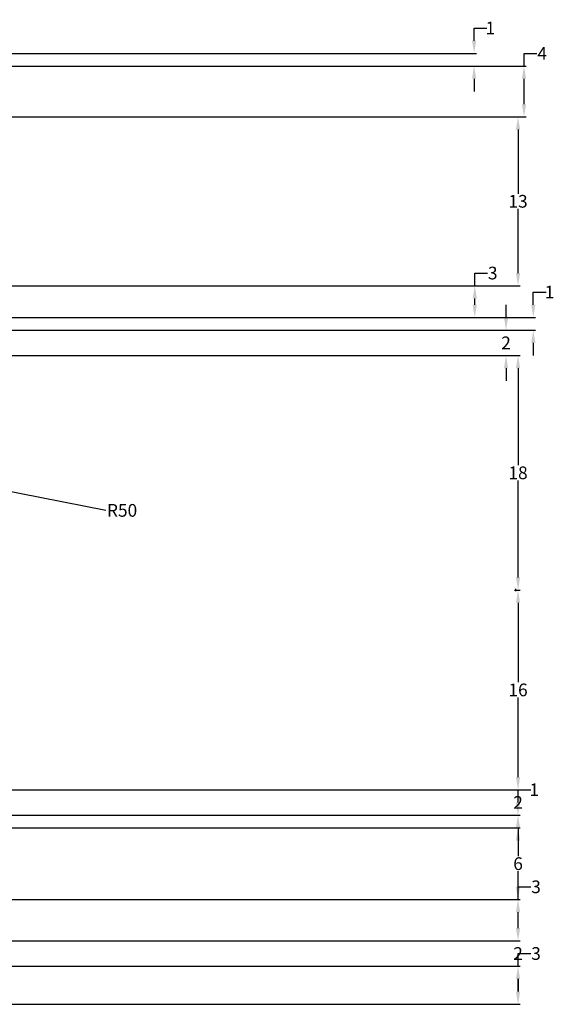
# Model space of a CAD drawing. Units: millimetres. Extents: x 31 to 232, y 35 to 192.
# Tile 3 of 5: x 80 to 122, y 43 to 121. Entities that reach past the tile are written whole.
import ezdxf

# ---------------------------------------------------------------- set-up
doc = ezdxf.new("R2010")
doc.units = ezdxf.units.MM
doc.header["$MEASUREMENT"] = 0
doc.layers.add('M-DIMS', color=2, linetype='Continuous', lineweight=25)
doc.styles.get("Standard").update_dxf_attribs({"font": 'arial.ttf'})
doc.dimstyles.get("Standard").update_dxf_attribs({"dimtxt": 1, "dimasz": 1, "dimexe": 0.18, "dimexo": 0.0625, "dimgap": 0.09, "dimtad": 0, "dimtih": 1, "dimtoh": 1, "dimdec": 0, "dimzin": 0, "dimdsep": 46, "dimtxsty": 'Standard', "dimcen": 0.09, "dimadec": 0, "dimazin": 0, "dimtfac": 1, "dimtdec": 0, "dimtofl": 0, "dimtmove": 0, "dimatfit": 3, "dimfxl": 1, "dimtolj": 1, "dimtzin": 0, "dimarcsym": 0})

# ---------------------------------------------------------------- blocks, each defined once
blk = doc.blocks.new('*D4')
at = {"layer": 'Defpoints', "color": 0, "transparency": 16777216}
for p in [(78.774, 46.183), (119.423, 46.183), (78.774, 43.183)]:
    blk.add_point(p, dxfattribs=at)
at = {"layer": 'M-DIMS', "color": 0, "lineweight": -2, "transparency": 16777216}
for p, q in [((119.423, 46.183), (119.423, 47.183)), ((119.423, 47.183), (120.423, 47.183)), ((78.836, 46.183), (119.603, 46.183)), ((119.423, 44.183), (119.423, 45.183)), ((78.836, 43.183), (119.603, 43.183))]:
    blk.add_line(p, q, dxfattribs=at)
at = {"layer": 'M-DIMS', "color": 0, "transparency": 16777216}
for points in [[(119.256, 45.183), (119.589, 45.183), (119.423, 46.183)], [(119.256, 44.183), (119.589, 44.183), (119.423, 43.183)]]:
    blk.add_solid(points, dxfattribs=at)
at = {"layer": 'M-DIMS', "color": 0, "transparency": 16777216, "insert": (120.84, 47.183), "char_height": 1, "attachment_point": 5}
blk.add_mtext('\\A1;3', dxfattribs=at)
blk = doc.blocks.new('*D5')
at = {"layer": 'Defpoints', "color": 0, "transparency": 16777216}
for p in [(76.774, 48.183), (119.423, 48.183), (78.774, 46.183)]:
    blk.add_point(p, dxfattribs=at)
at = {"layer": 'M-DIMS', "color": 0, "lineweight": -2, "transparency": 16777216}
for p, q in [((119.423, 49.183), (119.423, 50.183)), ((76.836, 48.183), (119.603, 48.183)), ((78.836, 46.183), (119.603, 46.183)), ((119.423, 45.183), (119.423, 44.183))]:
    blk.add_line(p, q, dxfattribs=at)
at = {"layer": 'M-DIMS', "color": 0, "transparency": 16777216}
for points in [[(119.256, 49.183), (119.589, 49.183), (119.423, 48.183)], [(119.256, 45.183), (119.589, 45.183), (119.423, 46.183)]]:
    blk.add_solid(points, dxfattribs=at)
at = {"layer": 'M-DIMS', "color": 0, "transparency": 16777216, "insert": (119.423, 47.183), "char_height": 1, "attachment_point": 5}
blk.add_mtext('\\A1;2', dxfattribs=at)
blk = doc.blocks.new('*D6')
at = {"layer": 'Defpoints', "color": 0, "transparency": 16777216}
for p in [(77.735, 51.44), (119.423, 51.44), (76.774, 48.183)]:
    blk.add_point(p, dxfattribs=at)
at = {"layer": 'M-DIMS', "color": 0, "lineweight": -2, "transparency": 16777216}
for p, q in [((119.423, 51.44), (119.423, 52.44)), ((119.423, 52.44), (120.423, 52.44)), ((77.797, 51.44), (119.603, 51.44)), ((119.423, 49.183), (119.423, 50.44)), ((76.836, 48.183), (119.603, 48.183))]:
    blk.add_line(p, q, dxfattribs=at)
at = {"layer": 'M-DIMS', "color": 0, "transparency": 16777216}
for points in [[(119.256, 50.44), (119.589, 50.44), (119.423, 51.44)], [(119.256, 49.183), (119.589, 49.183), (119.423, 48.183)]]:
    blk.add_solid(points, dxfattribs=at)
at = {"layer": 'M-DIMS', "color": 0, "transparency": 16777216, "insert": (120.84, 52.44), "char_height": 1, "attachment_point": 5}
blk.add_mtext('\\A1;3', dxfattribs=at)
blk = doc.blocks.new('*D7')
at = {"layer": 'Defpoints', "color": 0, "transparency": 16777216}
for p in [(73.774, 57.083), (119.423, 57.083), (77.735, 51.44)]:
    blk.add_point(p, dxfattribs=at)
at = {"layer": 'M-DIMS', "color": 0, "lineweight": -2, "transparency": 16777216}
for p, q in [((73.836, 57.083), (119.603, 57.083)), ((119.423, 56.083), (119.423, 54.862)), ((119.423, 52.44), (119.423, 53.661)), ((77.797, 51.44), (119.603, 51.44))]:
    blk.add_line(p, q, dxfattribs=at)
at = {"layer": 'M-DIMS', "color": 0, "transparency": 16777216}
for points in [[(119.256, 56.083), (119.589, 56.083), (119.423, 57.083)], [(119.256, 52.44), (119.589, 52.44), (119.423, 51.44)]]:
    blk.add_solid(points, dxfattribs=at)
at = {"layer": 'M-DIMS', "color": 0, "transparency": 16777216, "insert": (119.423, 54.261), "char_height": 1, "attachment_point": 5}
blk.add_mtext('\\A1;6', dxfattribs=at)
blk = doc.blocks.new('*D8')
at = {"layer": 'Defpoints', "color": 0, "transparency": 16777216}
for p in [(73.774, 58.083), (119.423, 58.083), (73.774, 57.083)]:
    blk.add_point(p, dxfattribs=at)
at = {"layer": 'M-DIMS', "color": 0, "lineweight": -2, "transparency": 16777216}
for p, q in [((119.423, 59.083), (119.423, 60.083)), ((119.423, 60.083), (120.423, 60.083)), ((73.836, 58.083), (119.603, 58.083)), ((73.836, 57.083), (119.603, 57.083)), ((119.423, 56.083), (119.423, 55.083))]:
    blk.add_line(p, q, dxfattribs=at)
at = {"layer": 'M-DIMS', "color": 0, "transparency": 16777216}
for points in [[(119.256, 59.083), (119.589, 59.083), (119.423, 58.083)], [(119.256, 56.083), (119.589, 56.083), (119.423, 57.083)]]:
    blk.add_solid(points, dxfattribs=at)
at = {"layer": 'M-DIMS', "color": 0, "transparency": 16777216, "insert": (120.697, 60.083), "char_height": 1, "attachment_point": 5}
blk.add_mtext('\\A1;1', dxfattribs=at)
blk = doc.blocks.new('*D9')
at = {"layer": 'Defpoints', "color": 0, "transparency": 16777216}
for p in [(71.774, 60.083), (119.423, 60.083), (73.774, 58.083)]:
    blk.add_point(p, dxfattribs=at)
at = {"layer": 'M-DIMS', "color": 0, "lineweight": -2, "transparency": 16777216}
for p, q in [((119.423, 61.083), (119.423, 62.083)), ((71.836, 60.083), (119.603, 60.083)), ((73.836, 58.083), (119.603, 58.083)), ((119.423, 57.083), (119.423, 56.083))]:
    blk.add_line(p, q, dxfattribs=at)
at = {"layer": 'M-DIMS', "color": 0, "transparency": 16777216}
for points in [[(119.256, 61.083), (119.589, 61.083), (119.423, 60.083)], [(119.256, 57.083), (119.589, 57.083), (119.423, 58.083)]]:
    blk.add_solid(points, dxfattribs=at)
at = {"layer": 'M-DIMS', "color": 0, "transparency": 16777216, "insert": (119.423, 59.083), "char_height": 1, "attachment_point": 5}
blk.add_mtext('\\A1;2', dxfattribs=at)
blk = doc.blocks.new('*D10')
at = {"layer": 'Defpoints', "color": 0, "transparency": 16777216}
for p in [(119.236, 75.81), (119.423, 75.81), (71.774, 60.083)]:
    blk.add_point(p, dxfattribs=at)
at = {"layer": 'M-DIMS', "color": 0, "lineweight": -2, "transparency": 16777216}
for p, q in [((119.298, 75.81), (119.603, 75.81)), ((119.423, 74.81), (119.423, 68.547)), ((119.423, 61.083), (119.423, 67.346)), ((71.836, 60.083), (119.603, 60.083))]:
    blk.add_line(p, q, dxfattribs=at)
at = {"layer": 'M-DIMS', "color": 0, "transparency": 16777216}
for points in [[(119.256, 74.81), (119.589, 74.81), (119.423, 75.81)], [(119.256, 61.083), (119.589, 61.083), (119.423, 60.083)]]:
    blk.add_solid(points, dxfattribs=at)
at = {"layer": 'M-DIMS', "color": 0, "transparency": 16777216, "insert": (119.423, 67.946), "char_height": 1, "attachment_point": 5}
blk.add_mtext('\\A1;16', dxfattribs=at)
blk = doc.blocks.new('*D11')
at = {"layer": 'Defpoints', "color": 0, "transparency": 16777216}
for p in [(72.774, 94.283), (119.423, 94.283), (119.236, 75.81)]:
    blk.add_point(p, dxfattribs=at)
at = {"layer": 'M-DIMS', "color": 0, "lineweight": -2, "transparency": 16777216}
for p, q in [((72.836, 94.283), (119.603, 94.283)), ((119.423, 93.283), (119.423, 85.647)), ((119.423, 76.81), (119.423, 84.446)), ((119.298, 75.81), (119.603, 75.81))]:
    blk.add_line(p, q, dxfattribs=at)
at = {"layer": 'M-DIMS', "color": 0, "transparency": 16777216}
for points in [[(119.256, 93.283), (119.589, 93.283), (119.423, 94.283)], [(119.256, 76.81), (119.589, 76.81), (119.423, 75.81)]]:
    blk.add_solid(points, dxfattribs=at)
at = {"layer": 'M-DIMS', "color": 0, "transparency": 16777216, "insert": (119.423, 85.046), "char_height": 1, "attachment_point": 5}
blk.add_mtext('\\A1;18', dxfattribs=at)
blk = doc.blocks.new('*D12')
at = {"layer": 'Defpoints', "color": 0, "transparency": 16777216}
for p in [(72.774, 96.283), (118.478, 96.283), (72.774, 94.283)]:
    blk.add_point(p, dxfattribs=at)
at = {"layer": 'M-DIMS', "color": 0, "lineweight": -2, "transparency": 16777216}
for p, q in [((118.478, 97.283), (118.478, 98.283)), ((72.836, 96.283), (118.658, 96.283)), ((72.836, 94.283), (118.658, 94.283)), ((118.478, 93.283), (118.478, 92.283))]:
    blk.add_line(p, q, dxfattribs=at)
at = {"layer": 'M-DIMS', "color": 0, "transparency": 16777216}
for points in [[(118.312, 97.283), (118.645, 97.283), (118.478, 96.283)], [(118.312, 93.283), (118.645, 93.283), (118.478, 94.283)]]:
    blk.add_solid(points, dxfattribs=at)
at = {"layer": 'M-DIMS', "color": 0, "transparency": 16777216, "insert": (118.478, 95.283), "char_height": 1, "attachment_point": 5}
blk.add_mtext('\\A1;2', dxfattribs=at)
blk = doc.blocks.new('*D13')
at = {"layer": 'Defpoints', "color": 0, "transparency": 16777216}
for p in [(74.506, 97.283), (120.627, 97.283), (72.774, 96.283)]:
    blk.add_point(p, dxfattribs=at)
at = {"layer": 'M-DIMS', "color": 0, "lineweight": -2, "transparency": 16777216}
for p, q in [((120.627, 98.283), (120.627, 99.283)), ((120.627, 99.283), (121.627, 99.283)), ((74.568, 97.283), (120.807, 97.283)), ((72.836, 96.283), (120.807, 96.283)), ((120.627, 95.283), (120.627, 94.283))]:
    blk.add_line(p, q, dxfattribs=at)
at = {"layer": 'M-DIMS', "color": 0, "transparency": 16777216}
for points in [[(120.46, 98.283), (120.794, 98.283), (120.627, 97.283)], [(120.46, 95.283), (120.794, 95.283), (120.627, 96.283)]]:
    blk.add_solid(points, dxfattribs=at)
at = {"layer": 'M-DIMS', "color": 0, "transparency": 16777216, "insert": (121.901, 99.283), "char_height": 1, "attachment_point": 5}
blk.add_mtext('\\A1;1', dxfattribs=at)
blk = doc.blocks.new('*D14')
at = {"layer": 'Defpoints', "color": 0, "transparency": 16777216}
for p in [(77.006, 99.783), (116.013, 99.783), (74.506, 97.283)]:
    blk.add_point(p, dxfattribs=at)
at = {"layer": 'M-DIMS', "color": 0, "lineweight": -2, "transparency": 16777216}
for p, q in [((116.013, 99.783), (116.013, 100.783)), ((116.013, 100.783), (117.013, 100.783)), ((77.068, 99.783), (116.193, 99.783)), ((116.013, 98.283), (116.013, 98.783)), ((74.568, 97.283), (116.193, 97.283))]:
    blk.add_line(p, q, dxfattribs=at)
at = {"layer": 'M-DIMS', "color": 0, "transparency": 16777216}
for points in [[(115.846, 98.783), (116.18, 98.783), (116.013, 99.783)], [(115.846, 98.283), (116.18, 98.283), (116.013, 97.283)]]:
    blk.add_solid(points, dxfattribs=at)
at = {"layer": 'M-DIMS', "color": 0, "transparency": 16777216, "insert": (117.43, 100.783), "char_height": 1, "attachment_point": 5}
blk.add_mtext('\\A1;3', dxfattribs=at)
blk = doc.blocks.new('*D15')
at = {"layer": 'Defpoints', "color": 0, "transparency": 16777216}
for p in [(77.006, 113.083), (119.423, 113.083), (77.006, 99.783)]:
    blk.add_point(p, dxfattribs=at)
at = {"layer": 'M-DIMS', "color": 0, "lineweight": -2, "transparency": 16777216}
for p, q in [((77.068, 113.083), (119.603, 113.083)), ((119.423, 112.083), (119.423, 107.034)), ((119.423, 100.783), (119.423, 105.832)), ((77.068, 99.783), (119.603, 99.783))]:
    blk.add_line(p, q, dxfattribs=at)
at = {"layer": 'M-DIMS', "color": 0, "transparency": 16777216}
for points in [[(119.256, 112.083), (119.589, 112.083), (119.423, 113.083)], [(119.256, 100.783), (119.589, 100.783), (119.423, 99.783)]]:
    blk.add_solid(points, dxfattribs=at)
at = {"layer": 'M-DIMS', "color": 0, "transparency": 16777216, "insert": (119.423, 106.433), "char_height": 1, "attachment_point": 5}
blk.add_mtext('\\A1;13', dxfattribs=at)
blk = doc.blocks.new('*D16')
at = {"layer": 'Defpoints', "color": 0, "transparency": 16777216}
for p in [(76.506, 117.083), (119.892, 117.083), (77.006, 113.083)]:
    blk.add_point(p, dxfattribs=at)
at = {"layer": 'M-DIMS', "color": 0, "lineweight": -2, "transparency": 16777216}
for p, q in [((119.892, 117.083), (119.892, 118.083)), ((119.892, 118.083), (120.892, 118.083)), ((76.568, 117.083), (120.072, 117.083)), ((119.892, 114.083), (119.892, 116.083)), ((77.068, 113.083), (120.072, 113.083))]:
    blk.add_line(p, q, dxfattribs=at)
at = {"layer": 'M-DIMS', "color": 0, "transparency": 16777216}
for points in [[(119.726, 116.083), (120.059, 116.083), (119.892, 117.083)], [(119.726, 114.083), (120.059, 114.083), (119.892, 113.083)]]:
    blk.add_solid(points, dxfattribs=at)
at = {"layer": 'M-DIMS', "color": 0, "transparency": 16777216, "insert": (121.328, 118.083), "char_height": 1, "attachment_point": 5}
blk.add_mtext('\\A1;4', dxfattribs=at)
blk = doc.blocks.new('*D17')
at = {"layer": 'Defpoints', "color": 0, "transparency": 16777216}
for p in [(75.506, 118.083), (115.962, 118.083), (76.506, 117.083)]:
    blk.add_point(p, dxfattribs=at)
at = {"layer": 'M-DIMS', "color": 0, "lineweight": -2, "transparency": 16777216}
for p, q in [((115.962, 119.083), (115.962, 120.083)), ((115.962, 120.083), (116.962, 120.083)), ((75.568, 118.083), (116.142, 118.083)), ((76.568, 117.083), (116.142, 117.083)), ((115.962, 116.083), (115.962, 115.083))]:
    blk.add_line(p, q, dxfattribs=at)
at = {"layer": 'M-DIMS', "color": 0, "transparency": 16777216}
for points in [[(115.795, 119.083), (116.128, 119.083), (115.962, 118.083)], [(115.795, 116.083), (116.128, 116.083), (115.962, 117.083)]]:
    blk.add_solid(points, dxfattribs=at)
at = {"layer": 'M-DIMS', "color": 0, "transparency": 16777216, "insert": (117.236, 120.083), "char_height": 1, "attachment_point": 5}
blk.add_mtext('\\A1;1', dxfattribs=at)
blk = doc.blocks.new('*D23')
at = {"layer": 'Defpoints', "color": 0, "transparency": 16777216}
for p in [(70.155, 85.355), (119.236, 75.81)]:
    blk.add_point(p, dxfattribs=at)
at = {"layer": 'M-DIMS', "color": 0, "lineweight": -2, "transparency": 16777216}
blk.add_line((86.946, 82.089), (71.137, 85.164), dxfattribs=at)
at = {"layer": 'M-DIMS', "color": 0, "transparency": 16777216}
blk.add_solid([(71.169, 85.328), (71.105, 85), (70.155, 85.355)], dxfattribs=at)
at = {"layer": 'M-DIMS', "color": 0, "transparency": 16777216, "insert": (88.229, 82.089), "char_height": 1, "attachment_point": 5}
blk.add_mtext('\\A1;R50', dxfattribs=at)
blk = doc.blocks.new('*D48')
at = {"layer": 'Defpoints', "color": 0, "transparency": 16777216}
for p in [(69.257, 77.271), (119.236, 75.81)]:
    blk.add_point(p, dxfattribs=at)
at = {"layer": 'M-DIMS', "color": 0, "lineweight": -2, "transparency": 16777216}
for p, q in [((39.27, 78.148), (68.258, 77.3)), ((119.146, 75.81), (119.326, 75.81)), ((119.236, 75.72), (119.236, 75.9))]:
    blk.add_line(p, q, dxfattribs=at)
at = {"layer": 'M-DIMS', "color": 0, "transparency": 16777216}
blk.add_solid([(68.263, 77.467), (68.253, 77.134), (69.257, 77.271)], dxfattribs=at)
at = {"layer": 'M-DIMS', "color": 0, "transparency": 16777216, "insert": (36.904, 78.148), "char_height": 1, "attachment_point": 5}
blk.add_mtext('\\A1;2X R50', dxfattribs=at)

msp = doc.modelspace()

# ---------------------------------------------------------------- dimensions: what is measured, and where the dimension line sits
at = {"layer": 'M-DIMS'}
for base, p1, p2, picture, middle in [((115.9616, 118.0829), (76.5057, 117.0829), (75.5057, 118.0829), '*D17', (117.2358, 120.0829)), ((119.8924, 117.0829), (77.0057, 113.0829), (76.5057, 117.0829), '*D16', (121.3282, 118.0829)), ((118.4782, 96.2829), (72.7736, 94.2829), (72.7736, 96.2829), '*D12', (118.4782, 95.2829))]:
    dim = msp.add_linear_dim(base=base, p1=p1, p2=p2, angle=270, dimstyle='Standard', override={"dimclrd": 0, "dimclre": 0, "dimclrt": 0}, dxfattribs=at)
    dim.commit()
    dim.dimension.update_dxf_attribs({"geometry": picture, "text_midpoint": middle, "dimtype": 160})
for base, p1, p2, picture, middle in [((119.4225, 113.0829), (77.0057, 99.7829), (77.0057, 113.0829), '*D15', (119.4225, 106.4329)), ((116.0129246117, 99.7828853826), (74.5056541686, 97.2828853826), (77.0056541686, 99.7828853826), '*D14', (117.4303461669, 100.7828853826)), ((120.6271, 97.2829), (72.7736, 96.2829), (74.5057, 97.2829), '*D13', (121.9012, 99.2829)), ((119.4225, 94.2829), (119.2359, 75.8097), (72.7736, 94.2829), '*D11', (119.4225, 85.0463)), ((119.4225, 75.8097), (71.7736, 60.0829), (119.2359, 75.8097), '*D10', (119.4225, 67.9463)), ((119.4225, 60.0829), (73.7736, 58.0829), (71.7736, 60.0829), '*D9', (119.4225, 59.0829)), ((119.4225, 58.0829), (73.7736, 57.0829), (73.7736, 58.0829), '*D8', (120.6967, 60.0829)), ((119.4225, 57.0829), (77.7346, 51.44), (73.7736, 57.0829), '*D7', (119.4225, 54.2614)), ((119.4225, 51.44), (76.7736, 48.1829), (77.7346, 51.44), '*D6', (120.8399, 52.44)), ((119.4225, 48.1829), (78.7736, 46.1829), (76.7736, 48.1829), '*D5', (119.4225, 47.1829)), ((119.4225, 46.1829), (78.7736, 43.1829), (78.7736, 46.1829), '*D4', (120.8399, 47.1829))]:
    dim = msp.add_linear_dim(base=base, p1=p1, p2=p2, angle=270, dimstyle='Standard', override={"dimclrd": 0, "dimclre": 0, "dimclrt": 0}, dxfattribs=at)
    dim.commit()
    dim.dimension.update_dxf_attribs({"geometry": picture, "text_midpoint": middle})
dim = msp.add_radius_dim(center=(119.2359, 75.8097), mpoint=(70.1554, 85.3549), dimstyle='Standard', override={"dimclrd": 0, "dimclre": 0, "dimclrt": 0}, dxfattribs=at)
dim.commit()
dim.dimension.update_dxf_attribs({"geometry": '*D23', "text_midpoint": (86.9462, 82.0894), "dimtype": 164})
dim = msp.add_radius_dim(center=(119.2359, 75.8097), mpoint=(69.2572, 77.271), text='2X <>', dimstyle='Standard', override={"dimdec": 0, "dimlfac": 1, "dimrnd": 0, "dimzin": 0, "dimdsep": 46, "dimlunit": 2}, dxfattribs=at)
dim.commit()
dim.dimension.update_dxf_attribs({"geometry": '*D48', "text_midpoint": (39.27, 78.1478), "dimtype": 164})

doc.saveas('drawing.dxf')
